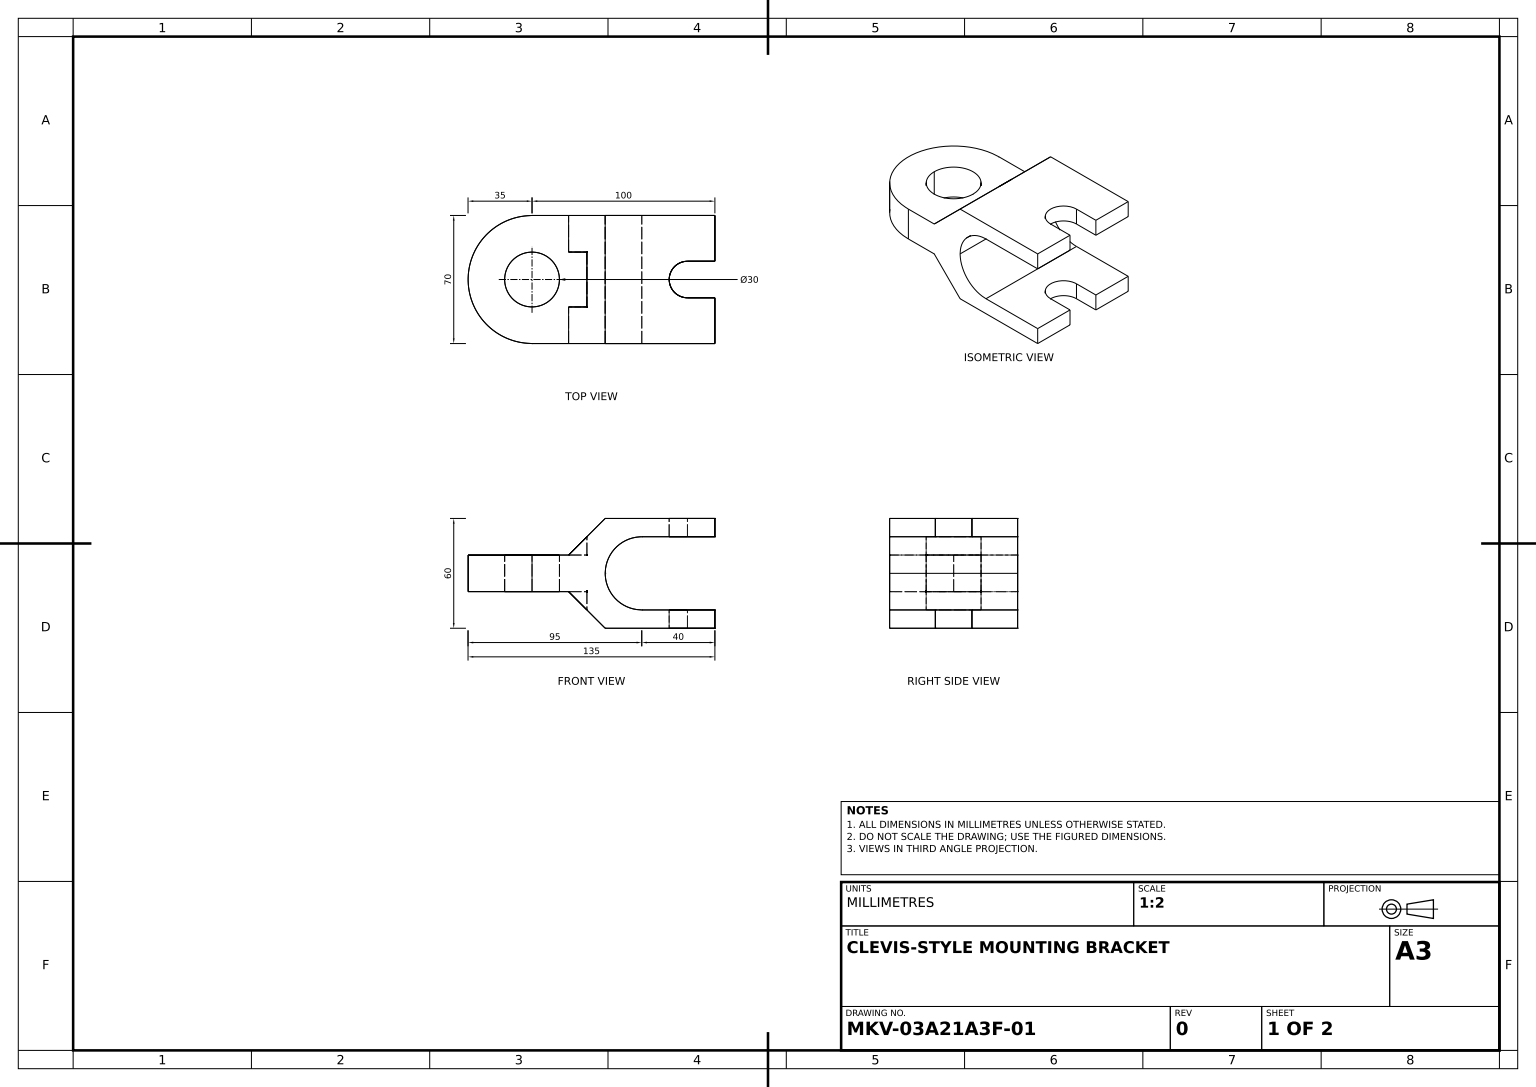
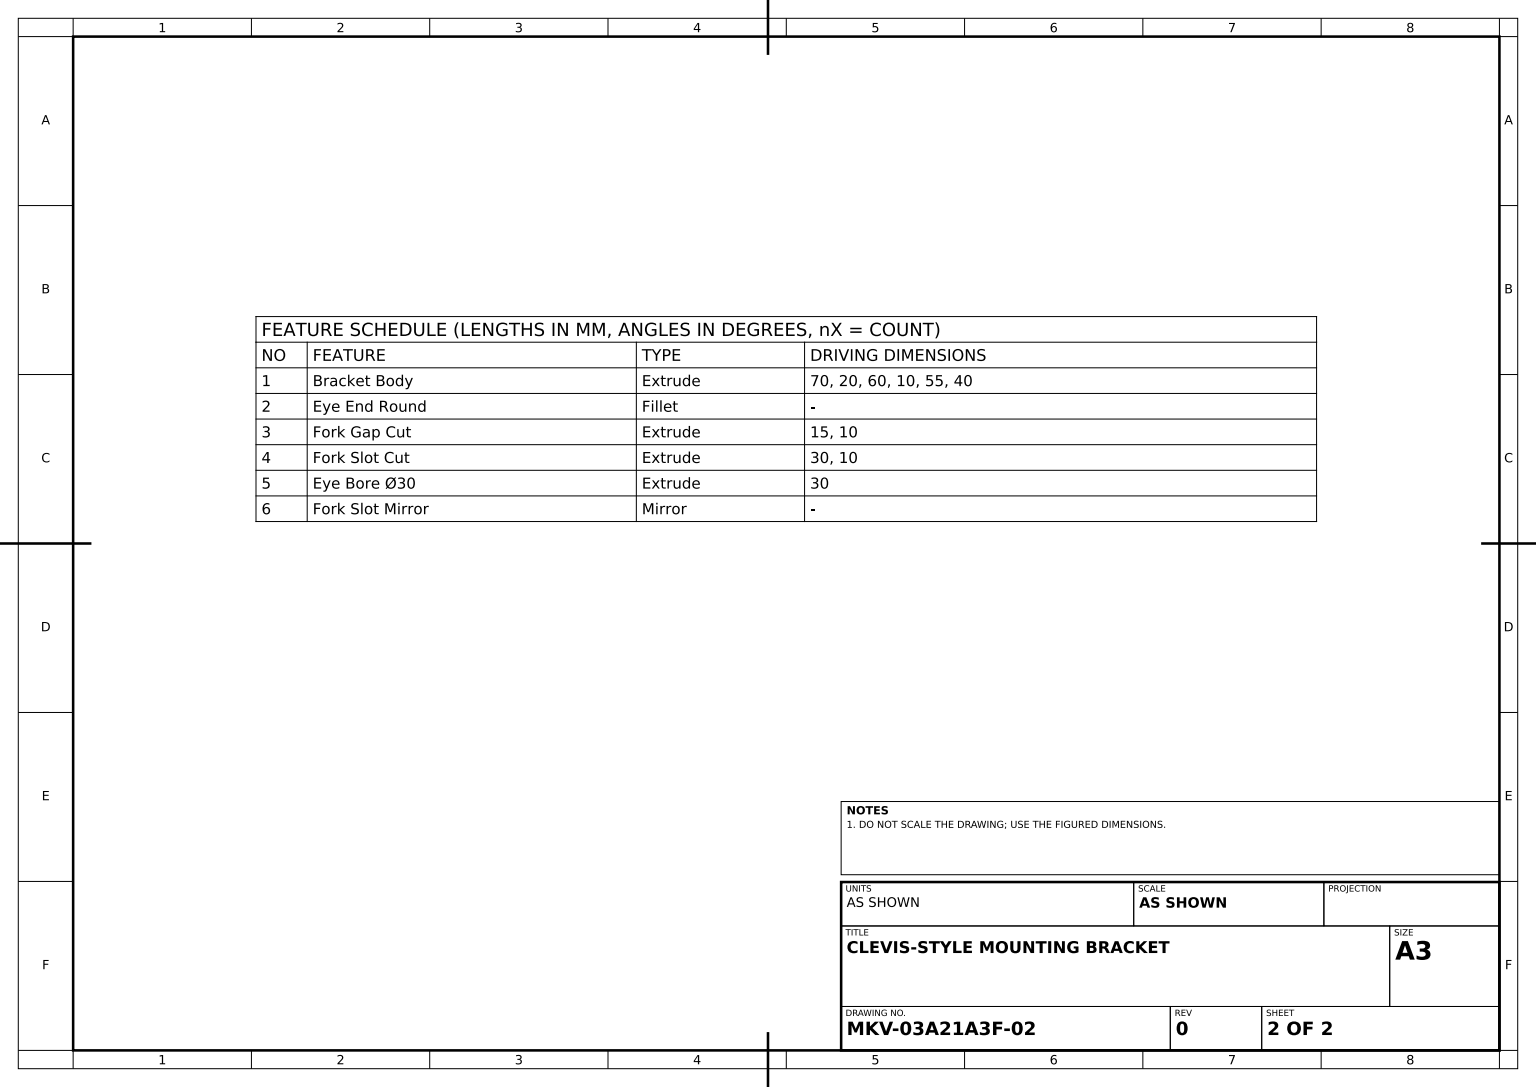
from build123d import *

# Parameters (mm, degrees)
BRACKET_BODY_DEPTH      = 35
EYE_END_ROUND_RADIUS    = 35
EYE_END_ROUND_LENGTH    = 20
FORK_GAP_CUT_DEPTH      = 106.59356041
FORK_GAP_CUT_DEPTH_BACK = 106.59356041
FORK_SLOT_CUT_DEPTH     = 15
EYE_BORE_30_REACH       = 110.858
EYE_BORE_SKETCH_R       = 15


with BuildPart() as part:
    # Bracket Profile Sketch → Bracket Body (new, symmetric)
    with BuildSketch(Plane.XY):
        with BuildLine():
            Line((40, -20), (0, -20))
            ThreePointArc((0, -20), (-20, 0), (0, 20))
            Line((0, 20), (40, 20))
            Line((40, 20), (40, 30))
            Line((40, 30), (-20, 30))
            Line((-20, 30), (-40, 10))
            Line((-40, 10), (-95, 10))
            Line((-95, 10), (-95, -10))
            Line((-95, -10), (-40, -10))
            Line((-40, -10), (-20, -30))
            Line((-20, -30), (40, -30))
            Line((40, -30), (40, -20))
        make_face()
    extrude(amount=BRACKET_BODY_DEPTH, both=True)

    # Eye End Round: full round fillet: the end face becomes a half cylinder, R = half its width
    eye_end_round_face = Plane((-95, 0, 0), x_dir=(0, -1, 0), z_dir=(-1, 0, 0))  # on the end face: x along it, z out of the body
    eye_end_round_slab = eye_end_round_face.offset(-EYE_END_ROUND_RADIUS / 2) * Box(EYE_END_ROUND_LENGTH, 2 * EYE_END_ROUND_RADIUS, EYE_END_ROUND_RADIUS, mode=Mode.PRIVATE)  # the body's end, R deep
    eye_end_round_round = Plane((-60, 0, 0), x_dir=(-1, 0, 0), z_dir=(0, -1, 0)) * Cylinder(EYE_END_ROUND_RADIUS, EYE_END_ROUND_LENGTH, mode=Mode.PRIVATE)  # its axis R under the face
    add(eye_end_round_slab - eye_end_round_round, mode=Mode.SUBTRACT)

    # Fork Gap Sketch → Fork Gap Cut (cut, two sides: drawn at the far end of the back side and taken through both)
    with BuildSketch(Plane(origin=(0, 0, 0), x_dir=(1, 0, 0), z_dir=(0, 1, 0)).offset(-FORK_GAP_CUT_DEPTH_BACK)):
        with BuildLine():
            Line((40, 10), (25, 10))
            ThreePointArc((25, 10), (15, 0), (25, -10))
            Line((25, -10), (40, -10))
            Line((40, -10), (40, 10))
        make_face()
    extrude(amount=FORK_GAP_CUT_DEPTH + FORK_GAP_CUT_DEPTH_BACK, mode=Mode.SUBTRACT)

    # Fork Slot Sketch → Fork Slot Cut (cut, symmetric)
    with BuildSketch(Plane.XY):
        Polygon((-40, 10), (-30, 10), (-30, 20), align=None)
    fork_slot_cut = extrude(amount=FORK_SLOT_CUT_DEPTH, both=True, mode=Mode.SUBTRACT)

    # Eye Bore Sketch → Eye Bore _30 (cut, up to next)
    with BuildSketch(Plane(origin=(0, 10, 0), x_dir=(1, 0, 0), z_dir=(0, 1, 0)), mode=Mode.PRIVATE) as eye_bore_30_sk1:
        with Locations(Location((-60, 0, 0), (0, 0, 180))):
            Circle(EYE_BORE_SKETCH_R)
    eye_bore_30_tool1 = extrude(eye_bore_30_sk1.sketch, amount=-EYE_BORE_30_REACH, mode=Mode.PRIVATE) & part.part
    add(eye_bore_30_tool1.solids().sort_by_distance((-60, 10, 0))[0], mode=Mode.SUBTRACT)

    # Fork Slot Mirror: Fork Slot Cut across plane
    add(fork_slot_cut.mirror(Plane.ZX), mode=Mode.SUBTRACT)


solid = part.part
